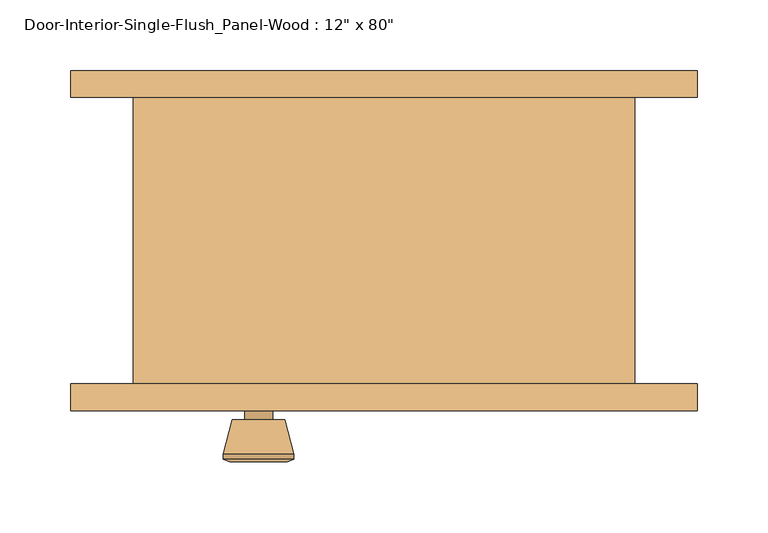
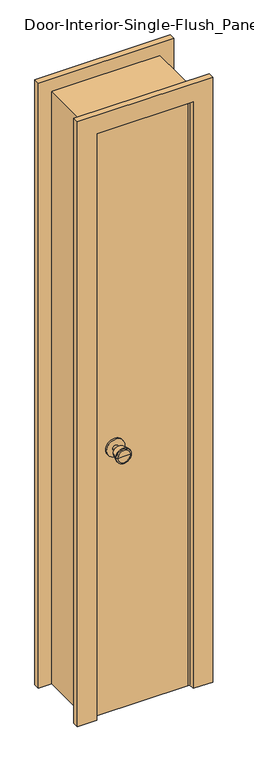
"""IFC4 building model written with IfcOpenShell, lengths in millimetres: door geometry."""

from ifc_helpers import new_model, si_unit, point, frame, frame_2d, origin, origin_with_axes, place, context, project, spatial, polyline, circle_curve, trimmed, segment, composite_curve, outline, extrude, faceted_brep, source, transform, mapped, element, save
from ifc_brep_helpers import plane_surface, cylinder_surface, revolved_surface, advanced_brep


def door_21b72c96(model_context):
    return source(origin(), model_context, "Body", "SolidModel", [
        advanced_brep(
        [(-88.9, -57.5, 914.4), (-98.9, -57.5, 914.4), (-78.9, -57.5, 914.4), (-68.4241324, -8.5, 914.4), (-109.3758676, -8.5, 914.4), (-88.9, -8.5, 914.4), (-63.9, -10.3278681, 914.4), (-113.9, -10.3278681, 914.4), (-63.9, -13.7915463, 914.4), (-113.9, -13.7915463, 914.4), (-70.263764, -38.5, 914.4), (-107.536236, -38.5, 914.4), (-78.9, -38.5, 914.4), (-98.9, -38.5, 914.4)],
        [
            (0, 1),
            (1, 2, circle_curve(frame((-88.9, -57.5, 914.4), z_axis=(0.0, -1.0, 0.0), x_axis=(-1.0, 0.0, 0.0)), 10.0)),
            (2, 0),
            (2, 1, circle_curve(frame((-88.9, -57.5, 914.4), z_axis=(0.0, -1.0, 0.0), x_axis=(-1.0, 0.0, 0.0)), 10.0)),
            (3, 4, circle_curve(frame((-88.9, -8.5, 914.4), z_axis=(0.0, 1.0, 0.0), x_axis=(-1.0, 0.0, 0.0)), 20.4758676)),
            (4, 5),
            (5, 3),
            (4, 3, circle_curve(frame((-88.9, -8.5, 914.4), z_axis=(0.0, 1.0, 0.0), x_axis=(-1.0, 0.0, 0.0)), 20.4758676)),
            (6, 7, circle_curve(frame((-88.9, -10.3278681, 914.4), z_axis=(0.0, 1.0, 0.0), x_axis=(-1.0, 0.0, 0.0)), 25.0)),
            (7, 4),
            (3, 6),
            (7, 6, circle_curve(frame((-88.9, -10.3278681, 914.4), z_axis=(0.0, 1.0, 0.0), x_axis=(-1.0, 0.0, 0.0)), 25.0)),
            (8, 9, circle_curve(frame((-88.9, -13.7915463, 914.4), z_axis=(0.0, 1.0, 0.0), x_axis=(-1.0, 0.0, 0.0)), 25.0)),
            (9, 7),
            (6, 8),
            (9, 8, circle_curve(frame((-88.9, -13.7915463, 914.4), z_axis=(0.0, 1.0, 0.0), x_axis=(-1.0, 0.0, 0.0)), 25.0)),
            (10, 11, circle_curve(frame((-88.9, -38.5, 914.4), z_axis=(0.0, 1.0, 0.0), x_axis=(-1.0, 0.0, 0.0)), 18.636236)),
            (11, 9),
            (8, 10),
            (11, 10, circle_curve(frame((-88.9, -38.5, 914.4), z_axis=(0.0, 1.0, 0.0), x_axis=(-1.0, 0.0, 0.0)), 18.636236)),
            (12, 13, circle_curve(frame((-88.9, -38.5, 914.4), z_axis=(0.0, 1.0, 0.0), x_axis=(-1.0, 0.0, 0.0)), 10.0)),
            (13, 11),
            (10, 12),
            (13, 12, circle_curve(frame((-88.9, -38.5, 914.4), z_axis=(0.0, 1.0, 0.0), x_axis=(-1.0, 0.0, 0.0)), 10.0)),
            (1, 13),
            (12, 2),
        ],
        [
            plane_surface(frame((-88.9, -57.5, 914.4), z_axis=(0.0, -1.0, 0.0), x_axis=(-1.0, 0.0, 0.0))),
            plane_surface(frame((-88.9, -8.5, 914.4), z_axis=(0.0, 1.0, 0.0), x_axis=(-1.0, 0.0, 0.0))),
            revolved_surface(polyline([(-109.3758676, -8.5, 914.4), (-113.9, -10.3278681, 914.4)]), (-88.9, -57.5, 914.4), (0.0, -1.0, 0.0)),
            cylinder_surface(frame((-88.9, -57.5, 914.4), z_axis=(0.0, -1.0, 0.0), x_axis=(-1.0, 0.0, 0.0)), 25.0),
            revolved_surface(polyline([(-113.9, -13.7915463, 914.4), (-107.536236, -38.5, 914.4)]), (-88.9, -57.5, 914.4), (0.0, -1.0, 0.0)),
            plane_surface(frame((-88.9, -38.5, 914.4), z_axis=(0.0, -1.0, 0.0), x_axis=(-1.0, 0.0, 0.0))),
            cylinder_surface(frame((-88.9, -57.5, 914.4), z_axis=(0.0, -1.0, 0.0), x_axis=(-1.0, 0.0, 0.0)), 10.0),
        ],
        [
            (0, [[1, 2, 3]]),
            (0, [[-3, 4, -1]]),
            (1, [[5, 6, 7]]),
            (1, [[8, -7, -6]]),
            (2, [[9, 10, -5, 11]]),
            (2, [[12, -11, -8, -10]]),
            (3, [[13, 14, -9, 15]]),
            (3, [[16, -15, -12, -14]]),
            (4, [[17, 18, -13, 19]]),
            (4, [[20, -19, -16, -18]]),
            (5, [[21, 22, -17, 23]]),
            (5, [[24, -23, -20, -22]]),
            (6, [[-2, 25, -21, 26]]),
            (6, [[-4, -26, -24, -25]]),
        ],
    ),
        extrude(outline(composite_curve([segment(trimmed(circle_curve(frame_2d((914.4, -88.9)), 30.0), [point((914.4, -118.9))], [point((914.4, -58.9))], False, "CARTESIAN"), True, "CONTINUOUS"), segment(trimmed(circle_curve(frame_2d((914.4, -88.9)), 30.0), [point((914.4, -58.9))], [point((914.4, -118.9))], False, "CARTESIAN"), True, "CONTINUOUS")], self_intersect=False)), frame((0.0, -63.5, 0.0), z_axis=(0.0, 1.0, 0.0), x_axis=(0.0, 0.0, 1.0)), (0.0, 0.0, 1.0), 6.0),
        advanced_brep(
        [(-88.9, -104.425, 914.4), (-78.9, -104.425, 914.4), (-98.9, -104.425, 914.4), (-68.4241324, -153.425, 914.4), (-88.9, -153.425, 914.4), (-109.3758676, -153.425, 914.4), (-63.9, -151.5971319, 914.4), (-113.9, -151.5971319, 914.4), (-63.9, -148.1334537, 914.4), (-113.9, -148.1334537, 914.4), (-70.263764, -123.425, 914.4), (-107.536236, -123.425, 914.4), (-78.9, -123.425, 914.4), (-98.9, -123.425, 914.4)],
        [
            (0, 1),
            (1, 2, circle_curve(frame((-88.9, -104.425, 914.4), z_axis=(0.0, 1.0, 0.0), x_axis=(-1.0, 0.0, 0.0)), 10.0)),
            (2, 0),
            (2, 1, circle_curve(frame((-88.9, -104.425, 914.4), z_axis=(0.0, 1.0, 0.0), x_axis=(-1.0, 0.0, 0.0)), 10.0)),
            (3, 4),
            (4, 5),
            (5, 3, circle_curve(frame((-88.9, -153.425, 914.4), z_axis=(0.0, -1.0, 0.0), x_axis=(-1.0, 0.0, 0.0)), 20.4758676)),
            (3, 5, circle_curve(frame((-88.9, -153.425, 914.4), z_axis=(0.0, -1.0, 0.0), x_axis=(-1.0, 0.0, 0.0)), 20.4758676)),
            (6, 3),
            (5, 7),
            (7, 6, circle_curve(frame((-88.9, -151.5971319, 914.4), z_axis=(0.0, -1.0, 0.0), x_axis=(-1.0, 0.0, 0.0)), 25.0)),
            (6, 7, circle_curve(frame((-88.9, -151.5971319, 914.4), z_axis=(0.0, -1.0, 0.0), x_axis=(-1.0, 0.0, 0.0)), 25.0)),
            (8, 6),
            (7, 9),
            (9, 8, circle_curve(frame((-88.9, -148.1334537, 914.4), z_axis=(0.0, -1.0, 0.0), x_axis=(-1.0, 0.0, 0.0)), 25.0)),
            (8, 9, circle_curve(frame((-88.9, -148.1334537, 914.4), z_axis=(0.0, -1.0, 0.0), x_axis=(-1.0, 0.0, 0.0)), 25.0)),
            (10, 8),
            (9, 11),
            (11, 10, circle_curve(frame((-88.9, -123.425, 914.4), z_axis=(0.0, -1.0, 0.0), x_axis=(-1.0, 0.0, 0.0)), 18.636236)),
            (10, 11, circle_curve(frame((-88.9, -123.425, 914.4), z_axis=(0.0, -1.0, 0.0), x_axis=(-1.0, 0.0, 0.0)), 18.636236)),
            (12, 10),
            (11, 13),
            (13, 12, circle_curve(frame((-88.9, -123.425, 914.4), z_axis=(0.0, -1.0, 0.0), x_axis=(-1.0, 0.0, 0.0)), 10.0)),
            (12, 13, circle_curve(frame((-88.9, -123.425, 914.4), z_axis=(0.0, -1.0, 0.0), x_axis=(-1.0, 0.0, 0.0)), 10.0)),
            (1, 12),
            (13, 2),
        ],
        [
            plane_surface(frame((-88.9, -104.425, 914.4), z_axis=(0.0, 1.0, 0.0), x_axis=(-1.0, 0.0, 0.0))),
            plane_surface(frame((-88.9, -153.425, 914.4), z_axis=(0.0, -1.0, 0.0), x_axis=(-1.0, 0.0, 0.0))),
            revolved_surface(polyline([(-109.3758676, -153.425, 914.4), (-113.9, -151.5971319, 914.4)]), (-88.9, -104.425, 914.4), (0.0, 1.0, 0.0)),
            cylinder_surface(frame((-88.9, -104.425, 914.4), z_axis=(0.0, 1.0, 0.0), x_axis=(-1.0, 0.0, 0.0)), 25.0),
            revolved_surface(polyline([(-113.9, -148.1334537, 914.4), (-107.536236, -123.425, 914.4)]), (-88.9, -104.425, 914.4), (0.0, 1.0, 0.0)),
            plane_surface(frame((-88.9, -123.425, 914.4), z_axis=(0.0, 1.0, 0.0), x_axis=(-1.0, 0.0, 0.0))),
            cylinder_surface(frame((-88.9, -104.425, 914.4), z_axis=(0.0, 1.0, 0.0), x_axis=(-1.0, 0.0, 0.0)), 10.0),
        ],
        [
            (0, [[1, 2, 3]]),
            (0, [[-3, 4, -1]]),
            (1, [[5, 6, 7]]),
            (1, [[-6, -5, 8]]),
            (2, [[9, -7, 10, 11]]),
            (2, [[-10, -8, -9, 12]]),
            (3, [[13, -11, 14, 15]]),
            (3, [[-14, -12, -13, 16]]),
            (4, [[17, -15, 18, 19]]),
            (4, [[-18, -16, -17, 20]]),
            (5, [[21, -19, 22, 23]]),
            (5, [[-22, -20, -21, 24]]),
            (6, [[25, -23, 26, -2]]),
            (6, [[-26, -24, -25, -4]]),
        ],
    ),
        extrude(outline(composite_curve([segment(trimmed(circle_curve(frame_2d((914.4, -88.9)), 30.0), [point((914.4, -118.9))], [point((914.4, -58.9))], False, "CARTESIAN"), True, "CONTINUOUS"), segment(trimmed(circle_curve(frame_2d((914.4, -88.9)), 30.0), [point((914.4, -58.9))], [point((914.4, -118.9))], False, "CARTESIAN"), True, "CONTINUOUS")], self_intersect=False)), frame((0.0, -104.425, 0.0), z_axis=(0.0, 1.0, 0.0), x_axis=(0.0, 0.0, 1.0)), (0.0, 0.0, 1.0), 6.0),
        extrude(outline(polyline([(152.4, -63.5), (152.4, -98.425), (-152.4, -98.425), (-152.4, -63.5), (152.4, -63.5)])), origin_with_axes(), (0.0, 0.0, 1.0), 2032.0),
        faceted_brep([(177.8, -98.425, 0.0), (152.4, -98.425, 0.0), (152.4, -63.5, 0.0), (139.7, -63.5, 0.0), (139.7, -28.575, 0.0), (152.4, -28.575, 0.0), (152.4, 104.775, 0.0), (177.8, 104.775, 0.0), (177.8, 104.775, 2057.4), (177.8, -98.425, 2057.4), (152.4, 104.775, 2032.0), (-152.4, 104.775, 2032.0), (-152.4, 104.775, 0.0), (-177.8, 104.775, 0.0), (-177.8, 104.775, 2057.4), (152.4, -28.575, 2032.0), (139.7, -28.575, 2019.3), (-139.7, -28.575, 2019.3), (-139.7, -28.575, 0.0), (-152.4, -28.575, 0.0), (-152.4, -28.575, 2032.0), (139.7, -63.5, 2019.3), (152.4, -63.5, 2032.0), (-152.4, -63.5, 2032.0), (-152.4, -63.5, 0.0), (-139.7, -63.5, 0.0), (-139.7, -63.5, 2019.3), (152.4, -98.425, 2032.0), (-177.8, -98.425, 2057.4), (-177.8, -98.425, 0.0), (-152.4, -98.425, 0.0), (-152.4, -98.425, 2032.0)], [[[0, 1, 2, 3, 4, 5, 6, 7]], [[7, 8, 9, 0]], [[6, 10, 11, 12, 13, 14, 8, 7]], [[5, 15, 10, 6]], [[4, 16, 17, 18, 19, 20, 15, 5]], [[3, 21, 16, 4]], [[2, 22, 23, 24, 25, 26, 21, 3]], [[1, 27, 22, 2]], [[0, 9, 28, 29, 30, 31, 27, 1]], [[8, 14, 28, 9]], [[15, 20, 11, 10]], [[21, 26, 17, 16]], [[27, 31, 23, 22]], [[29, 13, 12, 19, 18, 25, 24, 30]], [[14, 13, 29, 28]], [[20, 19, 12, 11]], [[26, 25, 18, 17]], [[31, 30, 24, 23]]]),
        extrude(outline(polyline([(0.0, 222.25), (2101.85, 222.25), (2101.85, -222.25), (0.0, -222.25), (0.0, -158.75), (2038.35, -158.75), (2038.35, 158.75), (0.0, 158.75), (0.0, 222.25)])), frame((0.0, 104.775, 0.0), z_axis=(0.0, 1.0, 0.0), x_axis=(0.0, 0.0, 1.0)), (0.0, 0.0, 1.0), 19.05),
        extrude(outline(polyline([(0.0, 222.25), (2101.85, 222.25), (2101.85, -222.25), (0.0, -222.25), (0.0, -158.75), (2038.35, -158.75), (2038.35, 158.75), (0.0, 158.75), (0.0, 222.25)])), frame((0.0, -117.475, 0.0), z_axis=(0.0, 1.0, 0.0), x_axis=(0.0, 0.0, 1.0)), (0.0, 0.0, 1.0), 19.05),
    ])


if __name__ == "__main__":
    model = new_model("IFC4")
    model_context = context("Model", 3, world=origin())
    ifc_project = project(units=[si_unit("LENGTHUNIT", "METRE", prefix="MILLI")], contexts=[model_context])
    site = spatial("IfcSite", under=ifc_project)
    building = spatial("IfcBuilding", under=site)
    placement = place(None, origin())
    door_shape = door_21b72c96(model_context)
    element("IfcDoor", 1, ObjectType="Door-Interior-Single-Flush_Panel-Wood : 12\" x 80\"", at=placement, inside=building, context=model_context, shape_type="MappedRepresentation", body=[
        mapped(door_shape, transform((0.0, 0.0, 0.0), x_axis=(1.0, 0.0, 0.0), y_axis=(0.0, 1.0, 0.0), z_axis=(0.0, 0.0, 1.0))),
    ])
    save(model, "model.ifc")

# Revit data of these elements
# Type "Door-Interior-Single-Flush_Panel-Wood : 12\" x 80\""
#   Type Mark = "9"
#   Assembly Code = "C1020300"
#   Analytic Construction = "Wooden"
#   Thickness = 0' - 1 3/8"
#   Thermal Resistance (R) = 2.5876 (h·ft²·°F)/BTU
#   Swing Angle [instance default] = 90.00°
#   Rough Width = 1' - 2"
#   Rough Height = 6' - 9"
#   Height = 6' - 8"
#   Width = 1' - 0"
#   Heat Transfer Coefficient (U) = 0.3865 BTU/(h·ft²·°F)
#   Trim Material = Cherry
#   Panel Material = Cherry
#   Frame Material = Cherry
#   Door Handle Material = Aluminum
#   Visual Light Transmittance = 0
#   Solar Heat Gain Coefficient = 0
#   Wall Closure = (empty or 0)
#   Function = (empty or 0)
# Element 1 (IfcDoor, "Door-Interior-Single-Flush_Panel-Wood : 12\" x 80\"")
#   Materials on its faces: "Cherry", "Aluminum"
# Materials
#   "Cherry": class "Wood", colour RGB 226 177 128, transparency 0, Description = "Prunus Serotina", Cost = 0
#   "Aluminum": class "Metal", colour RGB 247 247 247, transparency 0, Description = "Aluminum 6061", Cost = 0
